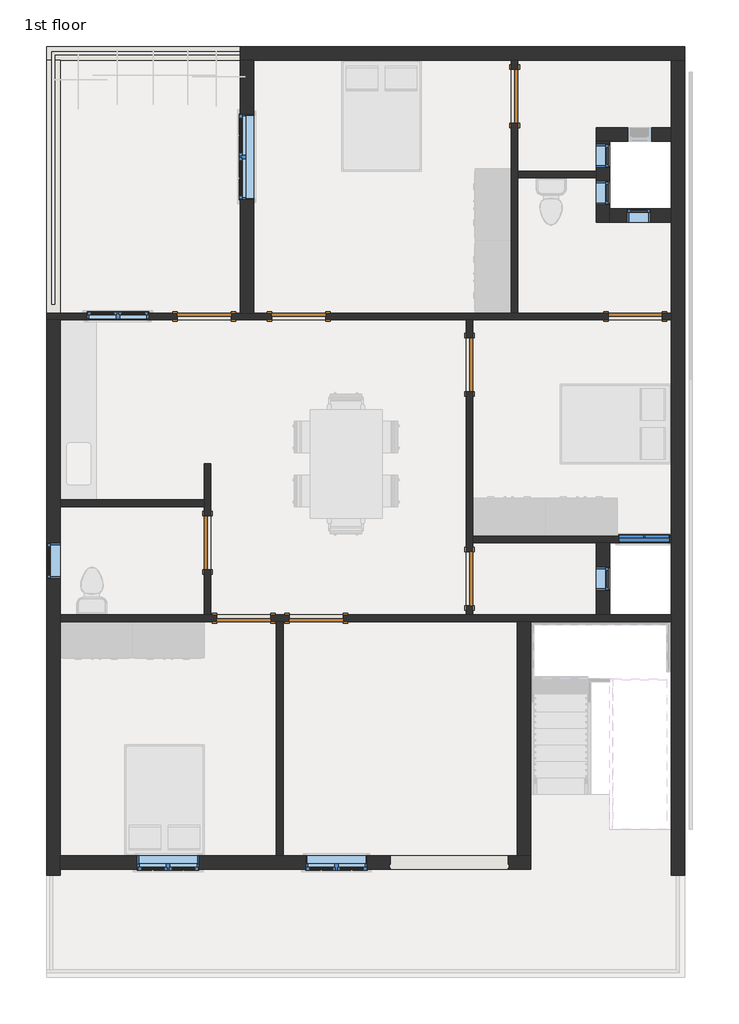
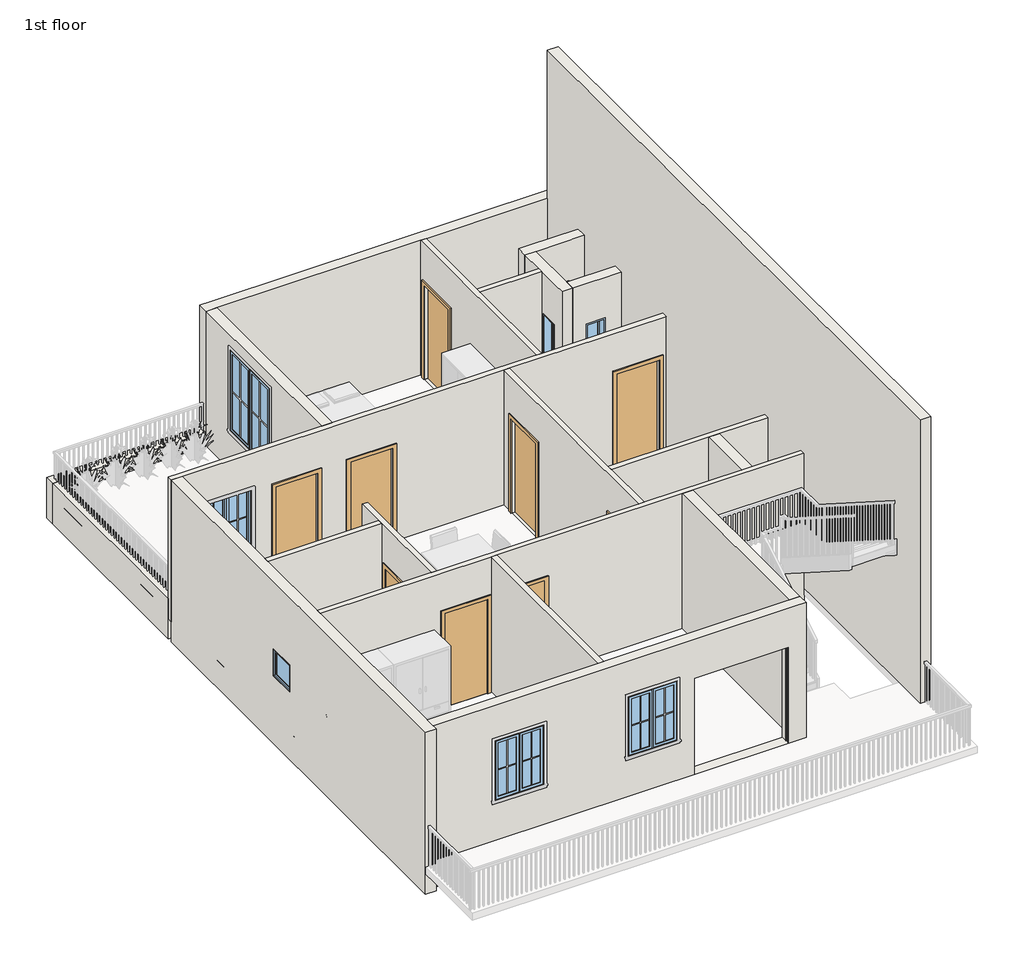
# One storey, part 1 of 5: 21 walls, 10 windows, 9 doors.
"""IFC4 building model written with IfcOpenShell, lengths in millimetres."""

from ifc_helpers import new_model, si_unit, frame, origin, place, context, project, spatial, polyline, outline, extrude, faceted_brep, transform, mapped, element, save
from components import door_305aa2a5, door_e5f9f3c4, window_aa618e30, window_cea7027f, window_80340324, window_a598f463, window_8ddb865a, window_c95ebb39, window_9ac97e1a

model = new_model("IFC4")

# Units and contexts
model_context = context("Model", 3, world=origin())
ifc_project = project(units=[si_unit("LENGTHUNIT", "METRE", prefix="MILLI")], contexts=[model_context])

# Site, building, storey
site = spatial("IfcSite", under=ifc_project)
building = spatial("IfcBuilding", under=site)
storey = spatial("IfcBuildingStorey", under=building, Name="1st floor", Elevation=3810.0)

# Doors
placement = place(None, origin())
door_shape = door_305aa2a5(model_context)
element("IfcDoor", 1, ObjectType="Single-Flush : 36\" x 84\"", at=placement, inside=storey, context=model_context, shape_type="MappedRepresentation", body=[
    mapped(door_shape, transform((-3843.1498597, 8241.1757925, 3810.0), x_axis=(-1.0, 0.0, 0.0), y_axis=(0.0, -1.0, 0.0), z_axis=(0.0, 0.0, 1.0))),
])
element("IfcDoor", 2, ObjectType="Single-Flush : 36\" x 84\"", at=placement, inside=storey, context=model_context, shape_type="MappedRepresentation", body=[
    mapped(door_shape, transform((-953.8998597, 7422.0257925, 3810.0), x_axis=(0.0, 1.0, 0.0), y_axis=(-1.0, 0.0, 0.0), z_axis=(0.0, 0.0, 1.0))),
])
element("IfcDoor", 3, ObjectType="Single-Flush : 36\" x 84\"", at=placement, inside=storey, context=model_context, shape_type="MappedRepresentation", body=[
    mapped(door_shape, transform((-4776.5998597, 3135.7757925, 3810.0), x_axis=(1.0, 0.0, 0.0), y_axis=(0.0, 1.0, 0.0), z_axis=(0.0, 0.0, 1.0))),
])
element("IfcDoor", 4, ObjectType="Single-Flush : 36\" x 84\"", at=placement, inside=storey, context=model_context, shape_type="MappedRepresentation", body=[
    mapped(door_shape, transform((-191.8998597, 11968.6257925, 3810.0), x_axis=(0.0, 1.0, 0.0), y_axis=(-1.0, 0.0, 0.0), z_axis=(0.0, 0.0, 1.0))),
])
door_2_shape = door_e5f9f3c4(model_context)
element("IfcDoor", 5, ObjectType="Single-Flush : 36\" x 84\"", at=placement, inside=storey, context=model_context, shape_type="MappedRepresentation", body=[
    mapped(door_2_shape, transform((1846.4501403, 8241.1757925, 3810.0), x_axis=(1.0, 0.0, 0.0), y_axis=(0.0, 1.0, 0.0), z_axis=(0.0, 0.0, 1.0))),
])
element("IfcDoor", 6, ObjectType="Single-Flush : 36\" x 84\"", at=placement, inside=storey, context=model_context, shape_type="MappedRepresentation", body=[
    mapped(door_2_shape, transform((-3551.0498597, 3135.7757925, 3810.0), x_axis=(-1.0, 0.0, 0.0), y_axis=(0.0, -1.0, 0.0), z_axis=(0.0, 0.0, 1.0))),
])
element("IfcDoor", 7, ObjectType="Single-Flush : 36\" x 84\"", at=placement, inside=storey, context=model_context, shape_type="MappedRepresentation", body=[
    mapped(door_2_shape, transform((-953.8998597, 3802.5257925, 3810.0), x_axis=(0.0, -1.0, 0.0), y_axis=(1.0, 0.0, 0.0), z_axis=(0.0, 0.0, 1.0))),
])
element("IfcDoor", 8, ObjectType="Single-Flush : 36\" x 84\"", at=placement, inside=storey, context=model_context, shape_type="MappedRepresentation", body=[
    mapped(door_2_shape, transform((-5443.3498597, 8241.1757925, 3810.0), x_axis=(1.0, 0.0, 0.0), y_axis=(0.0, 1.0, 0.0), z_axis=(0.0, 0.0, 1.0))),
])
element("IfcDoor", 9, ObjectType="Single-Flush : 36\" x 84\"", at=placement, inside=storey, context=model_context, shape_type="MappedRepresentation", body=[
    mapped(door_2_shape, transform((-5386.1998597, 4412.1257925, 3810.0), x_axis=(0.0, 1.0, 0.0), y_axis=(-1.0, 0.0, 0.0), z_axis=(0.0, 0.0, 1.0))),
])

# Walls
element("IfcWall", 10, at=placement, inside=storey, context=model_context, shape_type="Brep", body=[
    faceted_brep([(-8110.3498597, 12578.2257925, 3200.4), (-7881.7498597, 12578.2257925, 3200.4), (-4833.7498597, 12578.2257925, 3200.4), (-4833.7498597, 12578.2257925, 3657.6), (-4605.1498597, 12578.2257925, 3657.6), (-4605.1498597, 12578.2257925, 3810.0), (-4719.4498597, 12578.2257925, 3810.0), (-4719.4498597, 12578.2257925, 4114.8), (-4833.7498597, 12578.2257925, 4114.8), (-7881.7498597, 12578.2257925, 4114.8), (-8110.3498597, 12578.2257925, 4114.8), (-8110.3498597, 12806.8257925, 3200.4), (-8110.3498597, 12806.8257925, 4114.8), (-4833.7498597, 12806.8257925, 4114.8), (-4719.4498597, 12806.8257925, 4114.8), (-4719.4498597, 12806.8257925, 3810.0), (-4605.1498597, 12806.8257925, 3810.0), (-4605.1498597, 12806.8257925, 3657.6), (-4833.7498597, 12806.8257925, 3657.6), (-4833.7498597, 12806.8257925, 3200.4)], [[[0, 1, 2, 3, 4, 5, 6, 7, 8, 9, 10]], [[11, 12, 13, 14, 15, 16, 17, 18, 19]], [[2, 1, 0, 11, 19]], [[10, 9, 8, 7, 14, 13, 12]], [[0, 10, 12, 11]], [[17, 4, 3, 18]], [[3, 2, 19, 18]], [[7, 6, 15, 14]], [[15, 6, 5, 16]], [[5, 4, 17, 16]]]),
])
element("IfcWall", 11, at=placement, inside=storey, context=model_context, shape_type="Brep", body=[
    faceted_brep([(-4833.7498597, 12578.2257925, 6858.0), (-4833.7498597, 12578.2257925, 4114.8), (-4833.7498597, 12578.2257925, 3657.6), (-4833.7498597, 12578.2257925, 3200.4), (-4833.7498597, 8298.3257925, 3200.4), (-4833.7498597, 8298.3257925, 6858.0), (-4833.7498597, 11663.8257925, 6553.2), (-4833.7498597, 10216.0257925, 6553.2), (-4833.7498597, 10216.0257925, 4724.4), (-4833.7498597, 11663.8257925, 4724.4), (-4605.1498597, 12578.2257925, 3200.4), (-4605.1498597, 12578.2257925, 3657.6), (-4605.1498597, 12578.2257925, 3810.0), (-4605.1498597, 12578.2257925, 6858.0), (-4605.1498597, 8298.3257925, 6858.0), (-4605.1498597, 8298.3257925, 3200.4), (-4605.1498597, 11663.8257925, 6553.2), (-4605.1498597, 11663.8257925, 4724.4), (-4605.1498597, 10216.0257925, 4724.4), (-4605.1498597, 10216.0257925, 6553.2)], [[[0, 1, 2, 3, 4, 5], [6, 7, 8, 9]], [[10, 11, 12, 13, 14, 15], [16, 17, 18, 19]], [[4, 3, 10, 15]], [[17, 16, 6, 9]], [[18, 17, 9, 8]], [[19, 18, 8, 7]], [[16, 19, 7, 6]], [[4, 15, 14, 5]], [[0, 13, 12, 11, 10, 3, 2, 1]], [[0, 5, 14, 13]]]),
])
element("IfcWall", 12, at=placement, inside=storey, context=model_context, shape_type="Brep", body=[
    faceted_brep([(2456.0501403, 8298.3257925, 6858.0), (2456.0501403, 8298.3257925, 3200.4), (-134.7498597, 8298.3257925, 3200.4), (-249.0498597, 8298.3257925, 3200.4), (-4605.1498597, 8298.3257925, 3200.4), (-4833.7498597, 8298.3257925, 3200.4), (-7881.7498597, 8298.3257925, 3200.4), (-7881.7498597, 8298.3257925, 3657.6), (-8110.3498597, 8298.3257925, 3657.6), (-8110.3498597, 8298.3257925, 4114.8), (-8110.3498597, 8298.3257925, 6400.8), (-8110.3498597, 8298.3257925, 6858.0), (-7881.7498597, 8298.3257925, 6858.0), (-4833.7498597, 8298.3257925, 6858.0), (-4605.1498597, 8298.3257925, 6858.0), (-249.0498597, 8298.3257925, 6858.0), (-134.7498597, 8298.3257925, 6858.0), (1389.2501403, 8298.3257925, 3810.0), (2303.6501403, 8298.3257925, 3810.0), (2303.6501403, 8298.3257925, 5943.6), (1389.2501403, 8298.3257925, 5943.6), (-3385.9498597, 8298.3257925, 3810.0), (-3385.9498597, 8298.3257925, 5943.6), (-4300.3498597, 8298.3257925, 5943.6), (-4300.3498597, 8298.3257925, 3810.0), (-5900.5498597, 8298.3257925, 3810.0), (-4986.1498597, 8298.3257925, 3810.0), (-4986.1498597, 8298.3257925, 5943.6), (-5900.5498597, 8298.3257925, 5943.6), (-6383.1498597, 8298.3257925, 6070.6), (-7424.5498597, 8298.3257925, 6070.6), (-7424.5498597, 8298.3257925, 4724.4), (-6383.1498597, 8298.3257925, 4724.4), (2456.0501403, 8184.0257925, 3200.4), (2456.0501403, 8184.0257925, 6858.0), (-896.7498597, 8184.0257925, 6858.0), (-1011.0498597, 8184.0257925, 6858.0), (-7881.7498597, 8184.0257925, 6858.0), (-8110.3498597, 8184.0257925, 6858.0), (-8110.3498597, 8184.0257925, 6400.8), (-8110.3498597, 8184.0257925, 3657.6), (-7881.7498597, 8184.0257925, 3657.6), (-7881.7498597, 8184.0257925, 3200.4), (-1011.0498597, 8184.0257925, 3200.4), (-896.7498597, 8184.0257925, 3200.4), (1389.2501403, 8184.0257925, 3810.0), (1389.2501403, 8184.0257925, 5943.6), (2303.6501403, 8184.0257925, 5943.6), (2303.6501403, 8184.0257925, 3810.0), (-3385.9498597, 8184.0257925, 3810.0), (-4300.3498597, 8184.0257925, 3810.0), (-4300.3498597, 8184.0257925, 5943.6), (-3385.9498597, 8184.0257925, 5943.6), (-5900.5498597, 8184.0257925, 3810.0), (-5900.5498597, 8184.0257925, 5943.6), (-4986.1498597, 8184.0257925, 5943.6), (-4986.1498597, 8184.0257925, 3810.0), (-6383.1498597, 8184.0257925, 6070.6), (-6383.1498597, 8184.0257925, 4724.4), (-7424.5498597, 8184.0257925, 4724.4), (-7424.5498597, 8184.0257925, 6070.6)], [[[0, 1, 2, 3, 4, 5, 6, 7, 8, 9, 10, 11, 12, 13, 14, 15, 16], [17, 18, 19, 20], [21, 22, 23, 24], [25, 26, 27, 28], [29, 30, 31, 32]], [[33, 34, 35, 36, 37, 38, 39, 40, 41, 42, 43, 44], [45, 46, 47, 48], [49, 50, 51, 52], [53, 54, 55, 56], [57, 58, 59, 60]], [[6, 5, 4, 3, 2, 1, 33, 44, 43, 42]], [[18, 17, 45, 48]], [[19, 18, 48, 47]], [[20, 19, 47, 46]], [[17, 20, 46, 45]], [[50, 49, 21, 24]], [[51, 50, 24, 23]], [[52, 51, 23, 22]], [[49, 52, 22, 21]], [[26, 25, 53, 56]], [[27, 26, 56, 55]], [[28, 27, 55, 54]], [[25, 28, 54, 53]], [[58, 57, 29, 32]], [[59, 58, 32, 31]], [[60, 59, 31, 30]], [[57, 60, 30, 29]], [[40, 8, 7, 41]], [[7, 6, 42, 41]], [[8, 40, 39, 38, 11, 10, 9]], [[0, 16, 15, 14, 13, 12, 11, 38, 37, 36, 35, 34]], [[0, 34, 33, 1]]]),
])
element("IfcWall", 13, at=placement, inside=storey, context=model_context, shape_type="Brep", body=[
    faceted_brep([(2456.0501403, 11435.2257925, 6858.0), (2456.0501403, 11435.2257925, 3200.4), (1414.6501403, 11435.2257925, 3200.4), (1414.6501403, 11435.2257925, 3657.6), (1186.0501403, 11435.2257925, 3657.6), (1186.0501403, 11435.2257925, 6858.0), (1414.6501403, 11435.2257925, 6858.0), (1719.4501403, 11435.2257925, 5943.6), (1719.4501403, 11435.2257925, 4724.4), (2125.8501403, 11435.2257925, 4724.4), (2125.8501403, 11435.2257925, 5943.6), (2456.0501403, 11206.6257925, 3200.4), (2456.0501403, 11206.6257925, 6858.0), (1414.6501403, 11206.6257925, 6858.0), (1186.0501403, 11206.6257925, 6858.0), (1186.0501403, 11206.6257925, 6400.8), (1186.0501403, 11206.6257925, 3657.6), (1414.6501403, 11206.6257925, 3657.6), (1414.6501403, 11206.6257925, 3200.4), (1719.4501403, 11206.6257925, 5943.6), (2125.8501403, 11206.6257925, 5943.6), (2125.8501403, 11206.6257925, 4724.4), (1719.4501403, 11206.6257925, 4724.4)], [[[0, 1, 2, 3, 4, 5, 6], [7, 8, 9, 10]], [[11, 12, 13, 14, 15, 16, 17, 18], [19, 20, 21, 22]], [[2, 1, 11, 18]], [[8, 7, 19, 22]], [[9, 8, 22, 21]], [[10, 9, 21, 20]], [[7, 10, 20, 19]], [[16, 4, 3, 17]], [[3, 2, 18, 17]], [[4, 16, 15, 14, 5]], [[0, 6, 5, 14, 13, 12]], [[0, 12, 11, 1]]]),
])
element("IfcWall", 14, at=placement, inside=storey, context=model_context, shape_type="Brep", body=[
    faceted_brep([(1186.0501403, 11206.6257925, 3200.4), (1186.0501403, 10698.6257925, 3200.4), (1186.0501403, 10584.3257925, 3200.4), (1186.0501403, 10063.6257925, 3200.4), (1186.0501403, 10063.6257925, 3657.6), (1186.0501403, 9835.0257925, 3657.6), (1186.0501403, 9835.0257925, 6858.0), (1186.0501403, 10063.6257925, 6858.0), (1186.0501403, 10584.3257925, 6858.0), (1186.0501403, 10698.6257925, 6858.0), (1186.0501403, 11206.6257925, 6858.0), (1186.0501403, 11206.6257925, 3657.6), (1186.0501403, 10127.1257925, 5943.6), (1186.0501403, 10127.1257925, 4724.4), (1186.0501403, 10533.5257925, 4724.4), (1186.0501403, 10533.5257925, 5943.6), (1186.0501403, 10755.7299127, 5943.6), (1186.0501403, 10755.7299127, 4724.4), (1186.0501403, 11162.1299127, 4724.4), (1186.0501403, 11162.1299127, 5943.6), (1414.6501403, 10063.6257925, 3200.4), (1414.6501403, 11206.6257925, 3200.4), (1414.6501403, 11206.6257925, 6858.0), (1414.6501403, 11162.1299127, 6858.0), (1414.6501403, 10063.6257925, 6858.0), (1414.6501403, 9835.0257925, 6858.0), (1414.6501403, 9835.0257925, 6400.8), (1414.6501403, 9835.0257925, 3657.6), (1414.6501403, 10063.6257925, 3657.6), (1414.6501403, 10127.1257925, 4724.4), (1414.6501403, 10127.1257925, 5943.6), (1414.6501403, 10533.5257925, 5943.6), (1414.6501403, 10533.5257925, 4724.4), (1414.6501403, 10755.7299127, 4724.4), (1414.6501403, 10755.7299127, 5943.6), (1414.6501403, 11162.1299127, 5943.6), (1414.6501403, 11162.1299127, 4724.4)], [[[0, 1, 2, 3, 4, 5, 6, 7, 8, 9, 10, 11], [12, 13, 14, 15], [16, 17, 18, 19]], [[20, 21, 22, 23, 24, 25, 26, 27, 28], [29, 30, 31, 32], [33, 34, 35, 36]], [[3, 2, 1, 0, 21, 20]], [[13, 12, 30, 29]], [[14, 13, 29, 32]], [[15, 14, 32, 31]], [[12, 15, 31, 30]], [[16, 34, 33, 17]], [[17, 33, 36, 18]], [[34, 16, 19, 35]], [[35, 19, 18, 36]], [[5, 4, 28, 27]], [[4, 3, 20, 28]], [[21, 0, 11, 10, 22]], [[5, 27, 26, 25, 6]], [[22, 10, 9, 8, 7, 6, 25, 24, 23]]]),
])
element("IfcWall", 15, at=placement, inside=storey, context=model_context, shape_type="Brep", body=[
    faceted_brep([(1414.6501403, 9835.0257925, 6858.0), (1414.6501403, 9835.0257925, 3657.6), (1414.6501403, 9835.0257925, 3200.4), (2456.0501403, 9835.0257925, 3200.4), (2456.0501403, 9835.0257925, 6858.0), (2113.1501403, 9835.0257925, 5943.6), (2113.1501403, 9835.0257925, 4724.4), (1706.7501403, 9835.0257925, 4724.4), (1706.7501403, 9835.0257925, 5943.6), (1414.6501403, 10063.6257925, 3200.4), (1414.6501403, 10063.6257925, 6858.0), (2456.0501403, 10063.6257925, 6858.0), (2456.0501403, 10063.6257925, 3200.4), (2113.1501403, 10063.6257925, 5943.6), (1706.7501403, 10063.6257925, 5943.6), (1706.7501403, 10063.6257925, 4724.4), (2113.1501403, 10063.6257925, 4724.4)], [[[0, 1, 2, 3, 4], [5, 6, 7, 8]], [[9, 10, 11, 12], [13, 14, 15, 16]], [[3, 2, 9, 12]], [[6, 5, 13, 16]], [[7, 6, 16, 15]], [[8, 7, 15, 14]], [[5, 8, 14, 13]], [[0, 10, 9, 2, 1]], [[0, 4, 11, 10]], [[3, 12, 11, 4]]]),
])
element("IfcWall", 16, at=placement, inside=storey, context=model_context, shape_type="Brep", body=[
    faceted_brep([(-7881.7498597, 3078.6257925, 6858.0), (-7881.7498597, 3078.6257925, 3200.4), (-4224.1498597, 3078.6257925, 3200.4), (-4109.8498597, 3078.6257925, 3200.4), (-147.4498597, 3078.6257925, 3200.4), (81.1501403, 3078.6257925, 3200.4), (2456.0501403, 3078.6257925, 3200.4), (2456.0501403, 3078.6257925, 6858.0), (2430.6501403, 3078.6257925, 6858.0), (81.1501403, 3078.6257925, 6858.0), (-147.4498597, 3078.6257925, 6858.0), (-4109.8498597, 3078.6257925, 6858.0), (-4224.1498597, 3078.6257925, 6858.0), (-5233.7998597, 3078.6257925, 3810.0), (-5233.7998597, 3078.6257925, 5943.6), (-4319.3998597, 3078.6257925, 5943.6), (-4319.3998597, 3078.6257925, 3810.0), (-3093.8498597, 3078.6257925, 3810.0), (-4008.2498597, 3078.6257925, 3810.0), (-4008.2498597, 3078.6257925, 5943.6), (-3093.8498597, 3078.6257925, 5943.6), (-7881.7498597, 3192.9257925, 3200.4), (-7881.7498597, 3192.9257925, 6858.0), (-5443.3498597, 3192.9257925, 6858.0), (-5329.0498597, 3192.9257925, 6858.0), (-1011.0498597, 3192.9257925, 6858.0), (-896.7498597, 3192.9257925, 6858.0), (1186.0501403, 3192.9257925, 6858.0), (1414.6501403, 3192.9257925, 6858.0), (2456.0501403, 3192.9257925, 6858.0), (2456.0501403, 3192.9257925, 3200.4), (1414.6501403, 3192.9257925, 3200.4), (1186.0501403, 3192.9257925, 3200.4), (-896.7498597, 3192.9257925, 3200.4), (-1011.0498597, 3192.9257925, 3200.4), (-5329.0498597, 3192.9257925, 3200.4), (-5443.3498597, 3192.9257925, 3200.4), (-5233.7998597, 3192.9257925, 3810.0), (-4319.3998597, 3192.9257925, 3810.0), (-4319.3998597, 3192.9257925, 5943.6), (-5233.7998597, 3192.9257925, 5943.6), (-3093.8498597, 3192.9257925, 3810.0), (-3093.8498597, 3192.9257925, 5943.6), (-4008.2498597, 3192.9257925, 5943.6), (-4008.2498597, 3192.9257925, 3810.0)], [[[0, 1, 2, 3, 4, 5, 6, 7, 8, 9, 10, 11, 12], [13, 14, 15, 16], [17, 18, 19, 20]], [[21, 22, 23, 24, 25, 26, 27, 28, 29, 30, 31, 32, 33, 34, 35, 36], [37, 38, 39, 40], [41, 42, 43, 44]], [[6, 5, 4, 3, 2, 1, 21, 36, 35, 34, 33, 32, 31, 30]], [[38, 37, 13, 16]], [[39, 38, 16, 15]], [[40, 39, 15, 14]], [[37, 40, 14, 13]], [[18, 17, 41, 44]], [[19, 18, 44, 43]], [[20, 19, 43, 42]], [[17, 20, 42, 41]], [[0, 22, 21, 1]], [[0, 12, 11, 10, 9, 8, 7, 29, 28, 27, 26, 25, 24, 23, 22]], [[6, 30, 29, 7]]]),
])
element("IfcWall", 17, at=placement, inside=storey, context=model_context, shape_type="Brep", body=[
    faceted_brep([(-7881.7498597, -1112.3742075, 3200.4), (-147.4498597, -1112.3742075, 3200.4), (-147.4498597, -1112.3742075, 3657.6), (81.1501403, -1112.3742075, 3657.6), (81.1501403, -1112.3742075, 6858.0), (-147.4498597, -1112.3742075, 6858.0), (-7881.7498597, -1112.3742075, 6858.0), (-2299.8498597, -1112.3742075, 5979.5), (-299.8498597, -1112.3742075, 5979.5), (-299.8498597, -1112.3742075, 3810.0), (-2299.8498597, -1112.3742075, 3810.0), (-6573.6498597, -1112.3742075, 4724.4), (-6573.6498597, -1112.3742075, 6070.6), (-5532.2498597, -1112.3742075, 6070.6), (-5532.2498597, -1112.3742075, 4724.4), (-3725.5498597, -1112.3742075, 4724.4), (-3725.5498597, -1112.3742075, 6070.6), (-2684.1498597, -1112.3742075, 6070.6), (-2684.1498597, -1112.3742075, 4724.4), (-147.4498597, -883.7742075, 3200.4), (-4109.8498597, -883.7742075, 3200.4), (-4224.1498597, -883.7742075, 3200.4), (-7881.7498597, -883.7742075, 3200.4), (-7881.7498597, -883.7742075, 6858.0), (-4224.1498597, -883.7742075, 6858.0), (-4109.8498597, -883.7742075, 6858.0), (-147.4498597, -883.7742075, 6858.0), (81.1501403, -883.7742075, 6858.0), (81.1501403, -883.7742075, 6400.8), (81.1501403, -883.7742075, 3657.6), (-147.4498597, -883.7742075, 3657.6), (-299.8498597, -883.7742075, 5979.5), (-2299.8498597, -883.7742075, 5979.5), (-2299.8498597, -883.7742075, 3810.0), (-299.8498597, -883.7742075, 3810.0), (-6573.6498597, -883.7742075, 6070.6), (-6573.6498597, -883.7742075, 4724.4), (-5532.2498597, -883.7742075, 4724.4), (-5532.2498597, -883.7742075, 6070.6), (-3725.5498597, -883.7742075, 6070.6), (-3725.5498597, -883.7742075, 4724.4), (-2684.1498597, -883.7742075, 4724.4), (-2684.1498597, -883.7742075, 6070.6), (-2299.8498597, -1092.3742075, 5979.5), (-299.8498597, -1092.3742075, 5979.5), (-299.8498597, -1022.3742075, 5979.5), (-2299.8498597, -1022.3742075, 5979.5), (-2299.8498597, -1022.3742075, 3810.0), (-2314.8498597, -1022.3742075, 3810.0), (-2314.8498597, -1092.3742075, 3810.0), (-2299.8498597, -1092.3742075, 3810.0), (-299.8498597, -1092.3742075, 3810.0), (-284.8498597, -1092.3742075, 3810.0), (-284.8498597, -1022.3742075, 3810.0), (-299.8498597, -1022.3742075, 3810.0), (-284.8498597, -1022.3742075, 5994.5), (-2314.8498597, -1022.3742075, 5994.5), (-2314.8498597, -1092.3742075, 5994.5), (-284.8498597, -1092.3742075, 5994.5)], [[[0, 1, 2, 3, 4, 5, 6], [7, 8, 9, 10], [11, 12, 13, 14], [15, 16, 17, 18]], [[19, 20, 21, 22, 23, 24, 25, 26, 27, 28, 29, 30], [31, 32, 33, 34], [35, 36, 37, 38], [39, 40, 41, 42]], [[1, 0, 22, 21, 20, 19]], [[43, 44, 8, 7]], [[45, 46, 32, 31]], [[47, 48, 49, 50, 10, 9, 51, 52, 53, 54, 34, 33]], [[54, 45, 31, 34]], [[46, 47, 33, 32]], [[46, 45, 54, 53, 55, 56, 48, 47]], [[49, 48, 56, 57]], [[44, 43, 50, 49, 57, 58, 52, 51]], [[50, 43, 7, 10]], [[44, 51, 9, 8]], [[53, 52, 58, 55]], [[56, 55, 58, 57]], [[36, 35, 12, 11]], [[37, 36, 11, 14]], [[38, 37, 14, 13]], [[35, 38, 13, 12]], [[40, 39, 16, 15]], [[41, 40, 15, 18]], [[42, 41, 18, 17]], [[39, 42, 17, 16]], [[3, 2, 30, 29]], [[2, 1, 19, 30]], [[3, 29, 28, 27, 4]], [[22, 0, 6, 23]], [[6, 5, 4, 27, 26, 25, 24, 23]]]),
])
element("IfcWall", 18, at=placement, inside=storey, context=model_context, shape_type="SweptSolid", body=[
    extrude(outline(polyline([(-4109.8498597, 3078.6257925), (-4109.8498597, -883.7742075), (-4224.1498597, -883.7742075), (-4224.1498597, 3078.6257925), (-4109.8498597, 3078.6257925)])), frame((0.0, 0.0, 3200.4), z_axis=(0.0, 0.0, 1.0), x_axis=(1.0, 0.0, 0.0)), (0.0, 0.0, 1.0), 3657.6),
])
element("IfcWall", 19, at=placement, inside=storey, context=model_context, shape_type="Brep", body=[
    faceted_brep([(81.1501403, -883.7742075, 6858.0), (81.1501403, -883.7742075, 3657.6), (81.1501403, -883.7742075, 3200.4), (81.1501403, 3078.6257925, 3200.4), (81.1501403, 3078.6257925, 6858.0), (81.1501403, 157.6257925, 6858.0), (-147.4498597, -883.7742075, 3200.4), (-147.4498597, -883.7742075, 6858.0), (-147.4498597, 3078.6257925, 6858.0), (-147.4498597, 3078.6257925, 3200.4)], [[[0, 1, 2, 3, 4, 5]], [[6, 7, 8, 9]], [[3, 2, 6, 9]], [[0, 7, 6, 2, 1]], [[3, 9, 8, 4]], [[0, 5, 4, 8, 7]]]),
])
element("IfcWall", 20, at=placement, inside=storey, context=model_context, shape_type="SweptSolid", body=[
    extrude(outline(polyline([(3192.9257925, 3200.4), (3192.9257925, 6858.0), (4412.1257925, 6858.0), (4412.1257925, 3200.4), (3192.9257925, 3200.4)]), holes=[polyline([(3599.3257925, 5334.0), (3599.3257925, 4724.4), (4005.7257925, 4724.4), (4005.7257925, 5334.0), (3599.3257925, 5334.0)])]), frame((1186.0501403, 0.0, 0.0), z_axis=(1.0, 0.0, 0.0), x_axis=(0.0, 1.0, 0.0)), (0.0, 0.0, 1.0), 228.6),
])
element("IfcWall", 21, at=placement, inside=storey, context=model_context, shape_type="Brep", body=[
    faceted_brep([(-896.7498597, 3192.9257925, 6858.0), (-896.7498597, 3192.9257925, 3200.4), (-896.7498597, 4412.1257925, 3200.4), (-896.7498597, 4526.4257925, 3200.4), (-896.7498597, 8184.0257925, 3200.4), (-896.7498597, 8184.0257925, 6858.0), (-896.7498597, 4526.4257925, 6858.0), (-896.7498597, 4412.1257925, 6858.0), (-896.7498597, 6964.8257925, 3810.0), (-896.7498597, 6964.8257925, 5943.6), (-896.7498597, 7879.2257925, 5943.6), (-896.7498597, 7879.2257925, 3810.0), (-896.7498597, 4259.7257925, 3810.0), (-896.7498597, 3345.3257925, 3810.0), (-896.7498597, 3345.3257925, 5943.6), (-896.7498597, 4259.7257925, 5943.6), (-1011.0498597, 3192.9257925, 3200.4), (-1011.0498597, 3192.9257925, 6858.0), (-1011.0498597, 8184.0257925, 6858.0), (-1011.0498597, 8184.0257925, 3200.4), (-1011.0498597, 6964.8257925, 3810.0), (-1011.0498597, 7879.2257925, 3810.0), (-1011.0498597, 7879.2257925, 5943.6), (-1011.0498597, 6964.8257925, 5943.6), (-1011.0498597, 4259.7257925, 3810.0), (-1011.0498597, 4259.7257925, 5943.6), (-1011.0498597, 3345.3257925, 5943.6), (-1011.0498597, 3345.3257925, 3810.0)], [[[0, 1, 2, 3, 4, 5, 6, 7], [8, 9, 10, 11], [12, 13, 14, 15]], [[16, 17, 18, 19], [20, 21, 22, 23], [24, 25, 26, 27]], [[4, 3, 2, 1, 16, 19]], [[21, 20, 8, 11]], [[22, 21, 11, 10]], [[23, 22, 10, 9]], [[20, 23, 9, 8]], [[13, 12, 24, 27]], [[14, 13, 27, 26]], [[15, 14, 26, 25]], [[12, 15, 25, 24]], [[4, 19, 18, 5]], [[0, 17, 16, 1]], [[0, 7, 6, 5, 18, 17]]]),
])
element("IfcWall", 22, at=placement, inside=storey, context=model_context, shape_type="Brep", body=[
    faceted_brep([(-7881.7498597, -1213.9742075, 3200.4), (-7881.7498597, -1112.3742075, 3200.4), (-7881.7498597, -883.7742075, 3200.4), (-7881.7498597, 3078.6257925, 3200.4), (-7881.7498597, 3192.9257925, 3200.4), (-7881.7498597, 5021.7257925, 3200.4), (-7881.7498597, 5136.0257925, 3200.4), (-7881.7498597, 8184.0257925, 3200.4), (-7881.7498597, 8184.0257925, 6858.0), (-7881.7498597, 5136.0257925, 6858.0), (-7881.7498597, 5021.7257925, 6858.0), (-7881.7498597, 3192.9257925, 6858.0), (-7881.7498597, 3078.6257925, 6858.0), (-7881.7498597, -883.7742075, 6858.0), (-7881.7498597, -1112.3742075, 6858.0), (-7881.7498597, -1213.9742075, 6858.0), (-7881.7498597, 4412.1257925, 5334.0), (-7881.7498597, 4412.1257925, 4724.4), (-7881.7498597, 3802.5257925, 4724.4), (-7881.7498597, 3802.5257925, 5334.0), (-8110.3498597, -1213.9742075, 3200.4), (-8110.3498597, -1213.9742075, 6858.0), (-8110.3498597, 8184.0257925, 6858.0), (-8110.3498597, 8184.0257925, 3657.6), (-8110.3498597, 8184.0257925, 3200.4), (-8110.3498597, 4412.1257925, 5334.0), (-8110.3498597, 3802.5257925, 5334.0), (-8110.3498597, 3802.5257925, 4724.4), (-8110.3498597, 4412.1257925, 4724.4)], [[[0, 1, 2, 3, 4, 5, 6, 7, 8, 9, 10, 11, 12, 13, 14, 15], [16, 17, 18, 19]], [[20, 21, 22, 23, 24], [25, 26, 27, 28]], [[7, 6, 5, 4, 3, 2, 1, 0, 20, 24]], [[0, 15, 21, 20]], [[16, 19, 26, 25]], [[19, 18, 27, 26]], [[18, 17, 28, 27]], [[17, 16, 25, 28]], [[7, 24, 23, 22, 8]], [[15, 14, 13, 12, 11, 10, 9, 8, 22, 21]]]),
])
element("IfcWall", 23, at=placement, inside=storey, context=model_context, shape_type="Brep", body=[
    faceted_brep([(-7881.7498597, 8298.3257925, 4114.8), (-7881.7498597, 8298.3257925, 3200.4), (-7881.7498597, 12578.2257925, 3200.4), (-7881.7498597, 12578.2257925, 4114.8), (-8110.3498597, 8298.3257925, 3200.4), (-8110.3498597, 8298.3257925, 3657.6), (-8110.3498597, 8298.3257925, 4114.8), (-8110.3498597, 12578.2257925, 4114.8), (-8110.3498597, 12578.2257925, 3200.4)], [[[0, 1, 2, 3]], [[4, 5, 6, 7, 8]], [[2, 1, 4, 8]], [[0, 3, 7, 6]], [[3, 2, 8, 7]], [[0, 6, 5, 4, 1]]]),
])
element("IfcWall", 24, at=placement, inside=storey, context=model_context, shape_type="Brep", body=[
    faceted_brep([(-4719.4498597, 12578.2257925, 3810.0), (-4605.1498597, 12578.2257925, 3810.0), (2456.0501403, 12578.2257925, 3810.0), (2684.6501403, 12578.2257925, 3810.0), (2684.6501403, 12578.2257925, 6858.0), (-134.7498597, 12578.2257925, 6858.0), (-249.0498597, 12578.2257925, 6858.0), (-4605.1498597, 12578.2257925, 6858.0), (-4833.7498597, 12578.2257925, 6858.0), (-4833.7498597, 12578.2257925, 6400.8), (-4833.7498597, 12578.2257925, 4114.8), (-4719.4498597, 12578.2257925, 4114.8), (-4719.4498597, 12806.8257925, 3810.0), (-4719.4498597, 12806.8257925, 4114.8), (-4833.7498597, 12806.8257925, 4114.8), (-4833.7498597, 12806.8257925, 6400.8), (-4833.7498597, 12806.8257925, 6858.0), (-4605.1498597, 12806.8257925, 6858.0), (2684.6501403, 12806.8257925, 6858.0), (2684.6501403, 12806.8257925, 3810.0), (-4605.1498597, 12806.8257925, 3810.0)], [[[0, 1, 2, 3, 4, 5, 6, 7, 8, 9, 10, 11]], [[12, 13, 14, 15, 16, 17, 18, 19, 20]], [[3, 2, 1, 0, 12, 20, 19]], [[0, 11, 13, 12]], [[10, 14, 13, 11]], [[8, 16, 15, 14, 10, 9]], [[4, 3, 19, 18]], [[8, 7, 6, 5, 4, 18, 17, 16]]]),
])
element("IfcWall", 25, at=placement, inside=storey, context=model_context, shape_type="Brep", body=[
    faceted_brep([(2456.0501403, 12578.2257925, 10210.8), (2456.0501403, 12578.2257925, 3810.0), (2456.0501403, -1213.9742075, 3810.0), (2456.0501403, -1213.9742075, 10210.8), (2684.6501403, 12578.2257925, 3810.0), (2684.6501403, 12578.2257925, 6858.0), (2684.6501403, 12578.2257925, 7010.4), (2684.6501403, 12578.2257925, 10058.4), (2684.6501403, 12578.2257925, 10210.8), (2684.6501403, -1213.9742075, 10210.8), (2684.6501403, -1213.9742075, 3810.0)], [[[0, 1, 2, 3]], [[4, 5, 6, 7, 8, 9, 10]], [[2, 1, 4, 10]], [[3, 2, 10, 9]], [[0, 3, 9, 8]], [[0, 8, 7, 6, 5, 4, 1]]]),
])
element("IfcWall", 26, at=placement, inside=storey, context=model_context, shape_type="Brep", body=[
    faceted_brep([(-249.0498597, 12578.2257925, 6858.0), (-249.0498597, 12578.2257925, 3200.4), (-249.0498597, 8298.3257925, 3200.4), (-249.0498597, 8298.3257925, 6858.0), (-249.0498597, 11511.4257925, 3810.0), (-249.0498597, 12425.8257925, 3810.0), (-249.0498597, 12425.8257925, 5943.6), (-249.0498597, 11511.4257925, 5943.6), (-134.7498597, 12578.2257925, 3200.4), (-134.7498597, 12578.2257925, 6858.0), (-134.7498597, 10698.6257925, 6858.0), (-134.7498597, 10584.3257925, 6858.0), (-134.7498597, 8298.3257925, 6858.0), (-134.7498597, 8298.3257925, 3200.4), (-134.7498597, 10584.3257925, 3200.4), (-134.7498597, 10698.6257925, 3200.4), (-134.7498597, 11511.4257925, 3810.0), (-134.7498597, 11511.4257925, 5943.6), (-134.7498597, 12425.8257925, 5943.6), (-134.7498597, 12425.8257925, 3810.0)], [[[0, 1, 2, 3], [4, 5, 6, 7]], [[8, 9, 10, 11, 12, 13, 14, 15], [16, 17, 18, 19]], [[2, 1, 8, 15, 14, 13]], [[5, 4, 16, 19]], [[6, 5, 19, 18]], [[7, 6, 18, 17]], [[4, 7, 17, 16]], [[0, 3, 12, 11, 10, 9]], [[2, 13, 12, 3]], [[0, 9, 8, 1]]]),
])
element("IfcWall", 27, at=placement, inside=storey, context=model_context, shape_type="SweptSolid", body=[
    extrude(outline(polyline([(-134.7498597, 10698.6257925), (1186.0501403, 10698.6257925), (1186.0501403, 10584.3257925), (-134.7498597, 10584.3257925), (-134.7498597, 10698.6257925)])), frame((0.0, 0.0, 3200.4), z_axis=(0.0, 0.0, 1.0), x_axis=(1.0, 0.0, 0.0)), (0.0, 0.0, 1.0), 3657.6),
])
element("IfcWall", 28, at=placement, inside=storey, context=model_context, shape_type="Brep", body=[
    faceted_brep([(2456.0501403, 4526.4257925, 6858.0), (2456.0501403, 4526.4257925, 3200.4), (-896.7498597, 4526.4257925, 3200.4), (-896.7498597, 4526.4257925, 6858.0), (2430.6501403, 4526.4257925, 5029.2), (1567.0501403, 4526.4257925, 5029.2), (1567.0501403, 4526.4257925, 4114.8), (2430.6501403, 4526.4257925, 4114.8), (2456.0501403, 4412.1257925, 3200.4), (2456.0501403, 4412.1257925, 6858.0), (1414.6501403, 4412.1257925, 6858.0), (1186.0501403, 4412.1257925, 6858.0), (-896.7498597, 4412.1257925, 6858.0), (-896.7498597, 4412.1257925, 3200.4), (1186.0501403, 4412.1257925, 3200.4), (1414.6501403, 4412.1257925, 3200.4), (2430.6501403, 4412.1257925, 5029.2), (2430.6501403, 4412.1257925, 4114.8), (1567.0501403, 4412.1257925, 4114.8), (1567.0501403, 4412.1257925, 5029.2)], [[[0, 1, 2, 3], [4, 5, 6, 7]], [[8, 9, 10, 11, 12, 13, 14, 15], [16, 17, 18, 19]], [[2, 1, 8, 15, 14, 13]], [[17, 16, 4, 7]], [[18, 17, 7, 6]], [[19, 18, 6, 5]], [[16, 19, 5, 4]], [[0, 3, 12, 11, 10, 9]], [[0, 9, 8, 1]], [[2, 13, 12, 3]]]),
])
element("IfcWall", 29, at=placement, inside=storey, context=model_context, shape_type="SweptSolid", body=[
    extrude(outline(polyline([(-5443.3498597, 5021.7257925), (-7881.7498597, 5021.7257925), (-7881.7498597, 5136.0257925), (-5443.3498597, 5136.0257925), (-5443.3498597, 5021.7257925)])), frame((0.0, 0.0, 3200.4), z_axis=(0.0, 0.0, 1.0), x_axis=(1.0, 0.0, 0.0)), (0.0, 0.0, 1.0), 3657.6),
])
element("IfcWall", 30, at=placement, inside=storey, context=model_context, shape_type="Brep", body=[
    faceted_brep([(-5329.0498597, 3192.9257925, 6858.0), (-5329.0498597, 3192.9257925, 3200.4), (-5329.0498597, 5745.6257925, 3200.4), (-5329.0498597, 5745.6257925, 6858.0), (-5329.0498597, 3954.9257925, 3810.0), (-5329.0498597, 3954.9257925, 5943.6), (-5329.0498597, 4869.3257925, 5943.6), (-5329.0498597, 4869.3257925, 3810.0), (-5443.3498597, 3192.9257925, 3200.4), (-5443.3498597, 3192.9257925, 6858.0), (-5443.3498597, 5021.7257925, 6858.0), (-5443.3498597, 5136.0257925, 6858.0), (-5443.3498597, 5745.6257925, 6858.0), (-5443.3498597, 5745.6257925, 3200.4), (-5443.3498597, 5136.0257925, 3200.4), (-5443.3498597, 5021.7257925, 3200.4), (-5443.3498597, 3954.9257925, 3810.0), (-5443.3498597, 4869.3257925, 3810.0), (-5443.3498597, 4869.3257925, 5943.6), (-5443.3498597, 3954.9257925, 5943.6)], [[[0, 1, 2, 3], [4, 5, 6, 7]], [[8, 9, 10, 11, 12, 13, 14, 15], [16, 17, 18, 19]], [[2, 1, 8, 15, 14, 13]], [[3, 2, 13, 12]], [[17, 16, 4, 7]], [[18, 17, 7, 6]], [[19, 18, 6, 5]], [[16, 19, 5, 4]], [[0, 3, 12, 11, 10, 9]], [[0, 9, 8, 1]]]),
])

# Windows
window_shape = window_aa618e30(model_context)
element("IfcWindow", 31, ObjectType="Fixed : 16\" x 24\"", at=placement, inside=storey, context=model_context, shape_type="MappedRepresentation", body=[
    mapped(window_shape, transform((1300.3501403, 3764.4257925, 3810.0), x_axis=(0.0, -1.0, 0.0), y_axis=(1.0, 0.0, 0.0), z_axis=(0.0, 0.0, 1.0))),
])
window_2_shape = window_cea7027f(model_context)
element("IfcWindow", 32, ObjectType="Fixed : 16\" x 48\"", at=placement, inside=storey, context=model_context, shape_type="MappedRepresentation", body=[
    mapped(window_2_shape, transform((1948.0501403, 9949.3257925, 3810.0), x_axis=(1.0, 0.0, 0.0), y_axis=(0.0, 1.0, 0.0), z_axis=(0.0, 0.0, 1.0))),
])
element("IfcWindow", 33, ObjectType="Fixed : 16\" x 48\"", at=placement, inside=storey, context=model_context, shape_type="MappedRepresentation", body=[
    mapped(window_2_shape, transform((1300.3501403, 10292.2257925, 3810.0), x_axis=(0.0, -1.0, 0.0), y_axis=(1.0, 0.0, 0.0), z_axis=(0.0, 0.0, 1.0))),
])
element("IfcWindow", 34, ObjectType="Fixed : 16\" x 48\"", at=placement, inside=storey, context=model_context, shape_type="MappedRepresentation", body=[
    mapped(window_2_shape, transform((1300.3501403, 10920.8299127, 3810.0), x_axis=(0.0, -1.0, 0.0), y_axis=(1.0, 0.0, 0.0), z_axis=(0.0, 0.0, 1.0))),
])
window_3_shape = window_80340324(model_context)
element("IfcWindow", 35, ObjectType="Fixed : 24\" x 24\"", at=placement, inside=storey, context=model_context, shape_type="MappedRepresentation", body=[
    mapped(window_3_shape, transform((-7996.0498597, 4145.4257925, 3810.0), x_axis=(0.0, 1.0, 0.0), y_axis=(-1.0, 0.0, 0.0), z_axis=(0.0, 0.0, 1.0))),
])
window_4_shape = window_a598f463(model_context)
element("IfcWindow", 36, ObjectType="Window-Casement-Double : 34\" x 36\"", at=placement, inside=storey, context=model_context, shape_type="MappedRepresentation", body=[
    mapped(window_4_shape, transform((1998.8501403, 4469.2757925, 3200.4), x_axis=(1.0, 0.0, 0.0), y_axis=(0.0, 1.0, 0.0), z_axis=(0.0, 0.0, 1.0))),
])
window_5_shape = window_8ddb865a(model_context)
element("IfcWindow", 37, ObjectType="Window-Casement-Double : 41\" x 53\"", at=placement, inside=storey, context=model_context, shape_type="MappedRepresentation", body=[
    mapped(window_5_shape, transform((-6903.8498597, 8241.1757925, 3810.0), x_axis=(1.0, 0.0, 0.0), y_axis=(0.0, 1.0, 0.0), z_axis=(0.0, 0.0, 1.0))),
])
window_6_shape = window_c95ebb39(model_context)
element("IfcWindow", 38, ObjectType="Window-Casement-Double : 41\" x 53\"", at=placement, inside=storey, context=model_context, shape_type="MappedRepresentation", body=[
    mapped(window_6_shape, transform((-6052.9498597, -998.0742075, 3810.0), x_axis=(-1.0, 0.0, 0.0), y_axis=(0.0, -1.0, 0.0), z_axis=(0.0, 0.0, 1.0))),
])
element("IfcWindow", 39, ObjectType="Window-Casement-Double : 41\" x 53\"", at=placement, inside=storey, context=model_context, shape_type="MappedRepresentation", body=[
    mapped(window_6_shape, transform((-3204.8498597, -998.0742075, 3810.0), x_axis=(-1.0, 0.0, 0.0), y_axis=(0.0, -1.0, 0.0), z_axis=(0.0, 0.0, 1.0))),
])
window_7_shape = window_9ac97e1a(model_context)
element("IfcWindow", 40, ObjectType="Window-Casement-Double : 57\" x 72\"", at=placement, inside=storey, context=model_context, shape_type="MappedRepresentation", body=[
    mapped(window_7_shape, transform((-4719.4498597, 10939.9257925, 3810.0), x_axis=(0.0, 1.0, 0.0), y_axis=(-1.0, 0.0, 0.0), z_axis=(0.0, 0.0, 1.0))),
])

save(model, "model.ifc")

# Revit data of these elements
# Type "Single-Flush : 36\" x 84\""
#   Type Mark = "1"
#   Construction Type Id = "MDOOR"
#   Assembly Code = "C1020"
#   Analytic Construction = "Metal"
#   Thickness = 0' - 2"
#   Heat Transfer Coefficient (U) = 0.651978 BTU/(h·ft²·°F)
#   Height = 7' - 0"
#   Trim Projection Ext = 0' - 1"
#   Trim Projection Int = 0' - 1"
#   Trim Width = 0' - 3"
#   Width = 3' - 0"
#   Define Thermal Properties by = 1
#   Define Thermal Properties by = 1
#   Door Material = Door - Panel
#   Frame Material = Door - Frame
#   Visual Light Transmittance = 0
#   Solar Heat Gain Coefficient = 0
#   Function = (empty or 0)
#   Wall Closure = (empty or 0)
# Type
#   Assembly Code = "B2010"
#   Layers, outside or top first: 0' - 9" no material (function 1)
# Type
#   Assembly Code = "B2010"
#   Layers, outside or top first: 0' - 4 1/2" no material (function 1)
# Type "Fixed : 16\" x 24\""
#   Type Mark = "4"
#   Construction Type Id = "GSP4R"
#   Assembly Code = "B2020100"
#   Analytic Construction = "1/8 in Pilkington single glazing"
#   Visual Light Transmittance = 0.9
#   Solar Heat Gain Coefficient = 0.78
#   Heat Transfer Coefficient (U) = 0.6496 BTU/(h·ft²·°F)
#   Height = 2' - 0"
#   Default Sill Height = 3' - 0"
#   Width = 1' - 4"
#   Window Inset = 0' - 0 3/4"
#   Define Thermal Properties by = 1
#   Define Thermal Properties by = 1
#   Glass Pane Material = Glass
#   Sash Material = Sash
#   Wall Closure = (empty or 0)
# Type "Fixed : 16\" x 48\""
#   Type Mark = "5"
#   Construction Type Id = "GSP4R"
#   Assembly Code = "B2020100"
#   Analytic Construction = "1/8 in Pilkington single glazing"
#   Visual Light Transmittance = 0.9
#   Solar Heat Gain Coefficient = 0.78
#   Heat Transfer Coefficient (U) = 0.6496 BTU/(h·ft²·°F)
#   Height = 4' - 0"
#   Default Sill Height = 3' - 0"
#   Width = 1' - 4"
#   Window Inset = 0' - 0 3/4"
#   Define Thermal Properties by = 1
#   Define Thermal Properties by = 1
#   Glass Pane Material = Glass
#   Sash Material = Sash
#   Wall Closure = (empty or 0)
# Type "Fixed : 24\" x 24\""
#   Type Mark = "3"
#   Construction Type Id = "GSP4R"
#   Assembly Code = "B2020100"
#   Analytic Construction = "1/8 in Pilkington single glazing"
#   Visual Light Transmittance = 0.9
#   Solar Heat Gain Coefficient = 0.78
#   Heat Transfer Coefficient (U) = 0.6496 BTU/(h·ft²·°F)
#   Height = 2' - 0"
#   Default Sill Height = 3' - 0"
#   Width = 2' - 0"
#   Window Inset = 0' - 0 3/4"
#   Define Thermal Properties by = 1
#   Define Thermal Properties by = 1
#   Glass Pane Material = Glass
#   Sash Material = Sash
#   Wall Closure = (empty or 0)
# Type "Window-Casement-Double : 34\" x 36\""
#   Type Mark = "14"
#   Fire Rating = "0.5h"
#   Assembly Code = "B2020100"
#   Analytic Construction = "Double glazing - domestic"
#   Frame Extension [instance default] = 0' - 0 1/4"
#   Window Inset [instance default] = 0' - 0"
#   Wall Thickness [instance default] = 0' - 6"
#   Interior Wall Closure [instance default] = 0' - 2 1/4"
#   Half Width = 1' - 5"
#   Visual Light Transmittance = 0.81
#   Thermal Resistance (R) = 1.8146 (h·ft²·°F)/BTU
#   Solar Heat Gain Coefficient = 0.76
#   Rough Width = 2' - 10 1/2"
#   Rough Height = 3' - 0 1/2"
#   Height = 3' - 0"
#   Heat Transfer Coefficient (U) = 0.5511 BTU/(h·ft²·°F)
#   Exterior Wall Closure [instance default] = 0' - 1 1/4"
#   Extension Jamb [instance default] = 0' - 2 1/4"
#   Default Sill Height = 3' - 0"
#   Width = 2' - 10"
#   Define Thermal Properties by = 0
#   Muntin Visibility = yes
#   Interior Trim Visibility [instance default] = yes
#   Exterior Trim Visibility [instance default] = yes
#   Extension Jamb Visibility [instance default] = yes
#   Interior Trim Material = Wood - Stained
#   Muntin Pattern = Muntin Pattern_2x2 : Muntin Pattern_2x2
#   Interior Trim = Trim-Window-Interior-Flat : Picture Frame
#   Interior Frame Material = Wood - Stained
#   Glass Panel Material = Glass
#   Exterior Trim Material = Clad - White
#   Exterior Trim = Trim-Window-Exterior-Flat : with Sill
#   Exterior Frame Material = Clad - White
#   Wall Closure = (empty or 0)
# Type "Window-Casement-Double : 41\" x 53\""
#   Type Mark = "15"
#   Fire Rating = "0.5h"
#   Assembly Code = "B2020100"
#   Analytic Construction = "Double glazing - domestic"
#   Frame Extension [instance default] = 0' - 0 1/4"
#   Window Inset [instance default] = 0' - 0"
#   Wall Thickness [instance default] = 0' - 6"
#   Interior Wall Closure [instance default] = 0' - 2 1/4"
#   Half Width = 1' - 8 1/2"
#   Visual Light Transmittance = 0.81
#   Thermal Resistance (R) = 1.8146 (h·ft²·°F)/BTU
#   Solar Heat Gain Coefficient = 0.76
#   Rough Width = 3' - 5 1/2"
#   Rough Height = 4' - 5 1/2"
#   Height = 4' - 5"
#   Heat Transfer Coefficient (U) = 0.5511 BTU/(h·ft²·°F)
#   Exterior Wall Closure [instance default] = 0' - 1 1/4"
#   Extension Jamb [instance default] = 0' - 2 1/4"
#   Default Sill Height = 3' - 0"
#   Width = 3' - 5"
#   Define Thermal Properties by = 0
#   Muntin Visibility = yes
#   Interior Trim Visibility [instance default] = yes
#   Exterior Trim Visibility [instance default] = yes
#   Extension Jamb Visibility [instance default] = yes
#   Interior Trim Material = Wood - Stained
#   Muntin Pattern = Muntin Pattern_2x2 : Muntin Pattern_2x2
#   Interior Trim = Trim-Window-Interior-Flat : Picture Frame
#   Interior Frame Material = Wood - Stained
#   Glass Panel Material = Glass
#   Exterior Trim Material = Clad - White
#   Exterior Trim = Trim-Window-Exterior-Flat : with Sill
#   Exterior Frame Material = Clad - White
#   Wall Closure = (empty or 0)
# Type "Window-Casement-Double : 57\" x 72\""
#   Type Mark = "17"
#   Fire Rating = "0.5h"
#   Assembly Code = "B2020100"
#   Analytic Construction = "Double glazing - domestic"
#   Frame Extension [instance default] = 0' - 0 1/4"
#   Window Inset [instance default] = 0' - 0"
#   Wall Thickness [instance default] = 0' - 6"
#   Interior Wall Closure [instance default] = 0' - 2 1/4"
#   Half Width = 2' - 4 1/2"
#   Visual Light Transmittance = 0.81
#   Thermal Resistance (R) = 1.8146 (h·ft²·°F)/BTU
#   Solar Heat Gain Coefficient = 0.76
#   Rough Width = 4' - 9 1/2"
#   Rough Height = 6' - 0 1/2"
#   Height = 6' - 0"
#   Heat Transfer Coefficient (U) = 0.5511 BTU/(h·ft²·°F)
#   Exterior Wall Closure [instance default] = 0' - 1 1/4"
#   Extension Jamb [instance default] = 0' - 2 1/4"
#   Default Sill Height = 3' - 0"
#   Width = 4' - 9"
#   Define Thermal Properties by = 0
#   Muntin Visibility = yes
#   Interior Trim Visibility [instance default] = yes
#   Exterior Trim Visibility [instance default] = yes
#   Extension Jamb Visibility [instance default] = yes
#   Interior Trim Material = Wood - Stained
#   Muntin Pattern = Muntin Pattern_2x2 : Muntin Pattern_2x2
#   Interior Trim = Trim-Window-Interior-Flat : Picture Frame
#   Interior Frame Material = Wood - Stained
#   Glass Panel Material = Glass
#   Exterior Trim Material = Clad - White
#   Exterior Trim = Trim-Window-Exterior-Flat : with Sill
#   Exterior Frame Material = Clad - White
#   Wall Closure = (empty or 0)
# Elements 1, 2, 3, 4, 5, 6, 7, 8, 9 (IfcDoor, "Single-Flush : 36\" x 84\"")
#   Phase Created = New Construction
#   Materials on its faces: "Door - Frame", "Door - Panel"
# Elements 10, 23 (IfcWall)
#   built-in parameter 1001111 = -2' - 0"
#   Top Offset = 0' - 0"
#   Base Offset = -2' - 0"
#   Unconnected Height = 3' - 0"
#   wall height = 3' - 0"
#   Phase Created = New Construction
#   Base Constraint = 1st floor
#   Materials on its faces: "Default Wall"
# Elements 11, 12, 13, 14, 15, 16, 17, 18, 19, 20, 21, 22, 26, 27, 28, 29, 30 (IfcWall)
#   built-in parameter 1001111 = -2' - 0"
#   Top Offset = 0' - 0"
#   Base Offset = -2' - 0"
#   wall height = 12' - 0"
#   Phase Created = New Construction
#   Base Constraint = 1st floor
#   Top Constraint = 2nd floor
#   Materials on its faces: "Default Wall"
# Element 24 (IfcWall)
#   Top Offset = 0' - 0"
#   Base Offset = 0' - 0"
#   wall height = 10' - 0"
#   Phase Created = New Construction
#   Base Constraint = 1st floor
#   Top Constraint = 2nd floor
#   Materials on its faces: "Default Wall"
# Element 25 (IfcWall)
#   Top Offset = -3' - 6"
#   Base Offset = 0' - 0"
#   wall height = 21' - 0"
#   Phase Created = New Construction
#   Base Constraint = 1st floor
#   Top Constraint = parapet wall
#   Materials on its faces: "Default Wall"
# Element 31 (IfcWindow, "Fixed : 16\" x 24\"")
#   Mark = "21"
#   Phase Created = New Construction
#   Materials on its faces: "Sash", "Glass"
# Element 32 (IfcWindow, "Fixed : 16\" x 48\"")
#   Mark = "19"
#   Phase Created = New Construction
#   Materials on its faces: "Sash", "Glass"
# Element 33 (IfcWindow, "Fixed : 16\" x 48\"")
#   Mark = "23"
#   Phase Created = New Construction
#   Materials on its faces: "Sash", "Glass"
# Element 34 (IfcWindow, "Fixed : 16\" x 48\"")
#   Mark = "24"
#   Phase Created = New Construction
#   Materials on its faces: "Sash", "Glass"
# Element 35 (IfcWindow, "Fixed : 24\" x 24\"")
#   Mark = "22"
#   Phase Created = New Construction
#   Materials on its faces: "Sash", "Glass"
# Element 36 (IfcWindow, "Window-Casement-Double : 34\" x 36\"")
#   Mark = "40"
#   Window Inset = 0' - 0"
#   Interior Wall Closure = 0' - 2 1/4"
#   Frame Extension = 0' - 0 1/4"
#   Exterior Wall Closure = 0' - 1 1/4"
#   Interior Trim Visibility = yes
#   Exterior Trim Visibility = yes
#   Phase Created = New Construction
#   Materials on its faces: "Wood - Stained", "Glass", "Clad - White"
# Element 37 (IfcWindow, "Window-Casement-Double : 41\" x 53\"")
#   Mark = "16"
#   Window Inset = 0' - 0"
#   Interior Wall Closure = 0' - 2 1/4"
#   Frame Extension = 0' - 0 1/4"
#   Exterior Wall Closure = 0' - 1 1/4"
#   Interior Trim Visibility = yes
#   Exterior Trim Visibility = yes
#   Phase Created = New Construction
#   Materials on its faces: "Wood - Stained", "Glass", "Clad - White"
# Element 38 (IfcWindow, "Window-Casement-Double : 41\" x 53\"")
#   Mark = "17"
#   Window Inset = 0' - 0"
#   Interior Wall Closure = 0' - 2 1/4"
#   Frame Extension = 0' - 0 1/4"
#   Exterior Wall Closure = 0' - 1 1/4"
#   Interior Trim Visibility = yes
#   Exterior Trim Visibility = yes
#   Phase Created = New Construction
#   Materials on its faces: "Wood - Stained", "Glass", "Clad - White"
# Element 39 (IfcWindow, "Window-Casement-Double : 41\" x 53\"")
#   Mark = "18"
#   Window Inset = 0' - 0"
#   Interior Wall Closure = 0' - 2 1/4"
#   Frame Extension = 0' - 0 1/4"
#   Exterior Wall Closure = 0' - 1 1/4"
#   Interior Trim Visibility = yes
#   Exterior Trim Visibility = yes
#   Phase Created = New Construction
#   Materials on its faces: "Wood - Stained", "Glass", "Clad - White"
# Element 40 (IfcWindow, "Window-Casement-Double : 57\" x 72\"")
#   Mark = "15"
#   Window Inset = 0' - 0"
#   Interior Wall Closure = 0' - 2 1/4"
#   Frame Extension = 0' - 0 1/4"
#   Exterior Wall Closure = 0' - 1 1/4"
#   Interior Trim Visibility = yes
#   Exterior Trim Visibility = yes
#   Phase Created = New Construction
#   Materials on its faces: "Wood - Stained", "Glass", "Clad - White"
# Materials
#   "Door - Panel": class "Wood", colour RGB 210 159 95, transparency 0, Cost = 0
#   "Door - Frame": colour RGB 118 70 51, transparency 0, Cost = 0
#   "Glass": class "Glass", colour RGB 0 128 192, transparency 0.75, Description = "Soda Lime Glass", Cost = 0
#   "Sash": class "Wood", colour RGB 224 178 126, transparency 0, Cost = 0
#   "Wood - Stained": class "Wood", colour RGB 224 178 126, transparency 0, Cost = 0
#   "Clad - White": class "Wood", colour RGB 242 242 238, transparency 0, Cost = 0
#   "Default Wall": colour RGB 128 128 128, transparency 0, Cost = 0
# Area, not placed, upper offset 0' - 0", lower offset 0' - 0"
#   Number = "1"
#   Name = "Area"
